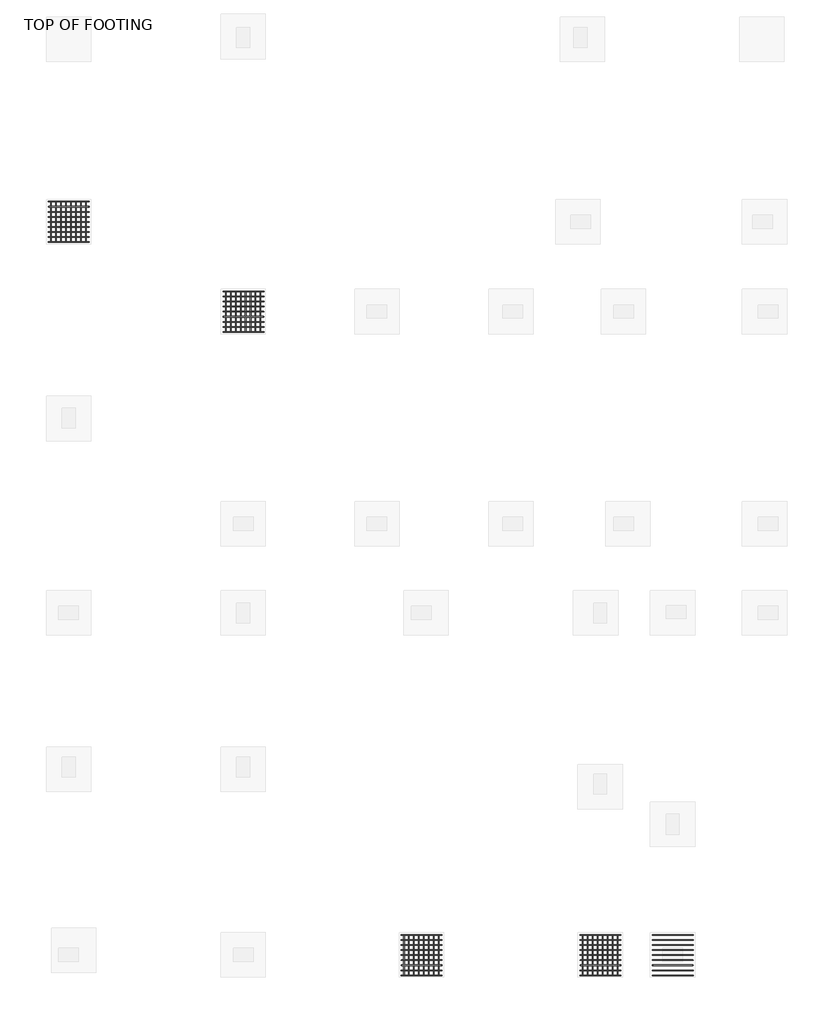
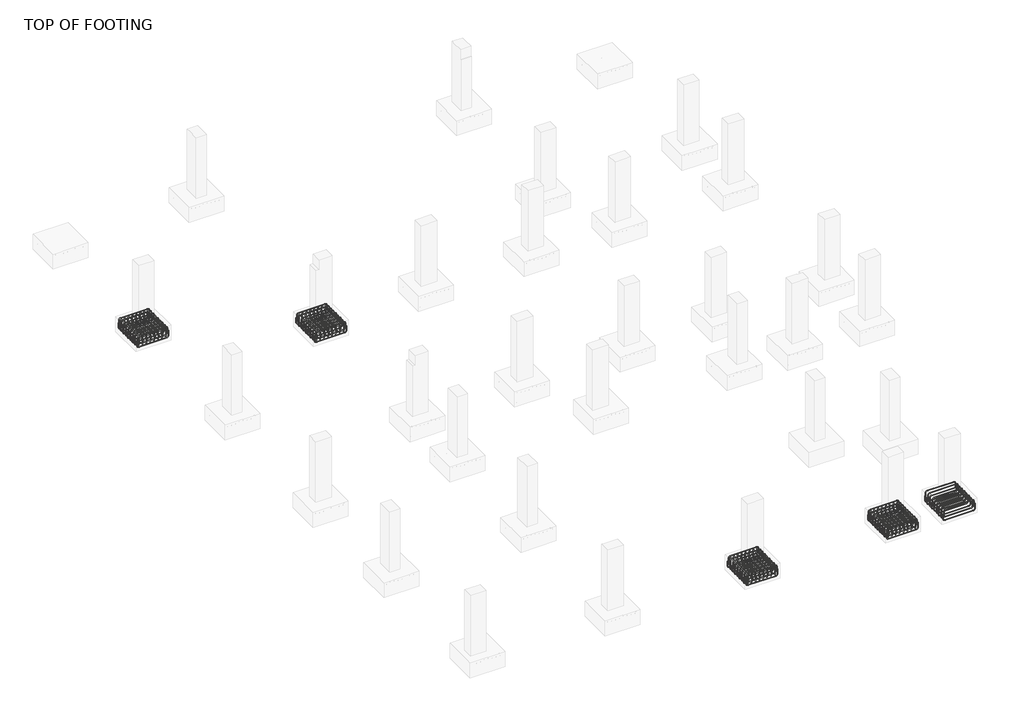
# One storey, part 5 of 20: 18 reinforcing bars.
"""IFC4 building model written with IfcOpenShell, lengths in millimetres."""

from ifc_helpers import new_model, si_unit, point, frame, origin, place, context, project, spatial, polyline, circle_curve, trimmed, segment, composite_curve, source, transform, mapped, element, save
from ifc_brep_helpers import swept_disk

model = new_model("IFC4")

# Units and contexts
model_context = context("Model", 3, world=origin())
ifc_project = project(units=[si_unit("LENGTHUNIT", "METRE", prefix="MILLI")], contexts=[model_context])

# Site, building, storey
site = spatial("IfcSite", under=ifc_project)
building = spatial("IfcBuilding", under=site)
storey = spatial("IfcBuildingStorey", under=building, Name="TOP OF FOOTING", Elevation=-1828.8)

# Reinforcing bars
placement = place(None, origin())
reinforcing_bar_shape = source(origin(), model_context, "Body", "SolidModel", [
    swept_disk(composite_curve([segment(polyline([(-1368.1365686, -4547.9729916, -2006.6587682), (-1368.1365686, -4547.9729916, -2153.9587682)]), True, "CONTINUOUS"), segment(trimmed(circle_curve(frame((-1414.4865686, -4547.9729916, -2153.9587682), z_axis=(0.0, 1.0, 0.0), x_axis=(46.350000000000136, 0.0, 0.0)), 46.35), [point((-1368.1365686, -4547.9729916, -2153.9587682))], [point((-1414.4865686, -4547.9729916, -2200.3087682))], True, "CARTESIAN"), True, "CONTINUOUS"), segment(polyline([(-1414.4865686, -4547.9729916, -2200.3087682), (-2229.0865686, -4547.9729916, -2200.3087682)]), True, "CONTINUOUS"), segment(trimmed(circle_curve(frame((-2229.0865686, -4547.9729916, -2153.9587682), z_axis=(0.0, 1.0, 0.0), x_axis=(0.0, 0.0, -46.34999999999991)), 46.35), [point((-2229.0865686, -4547.9729916, -2200.3087682))], [point((-2275.4365686, -4547.9729916, -2153.9587682))], True, "CARTESIAN"), True, "CONTINUOUS"), segment(polyline([(-2275.4365686, -4547.9729916, -2153.9587682), (-2275.4365686, -4547.9729916, -2006.6587682)]), True, "CONTINUOUS")], self_intersect=False), 6.35),
])
element("IfcReinforcingBar", 1, at=placement, inside=storey, context=model_context, shape_type="MappedRepresentation", body=[
    mapped(reinforcing_bar_shape, transform((0.0, 0.0, 0.0), x_axis=(1.0, 0.0, 0.0), y_axis=(0.0, 1.0, 0.0), z_axis=(0.0, 0.0, 1.0))),
    mapped(reinforcing_bar_shape, transform((0.0, -113.4125, 0.0), x_axis=(1.0, 0.0, 0.0), y_axis=(0.0, 1.0, 0.0), z_axis=(0.0, 0.0, 1.0))),
    mapped(reinforcing_bar_shape, transform((0.0, -226.825, 0.0), x_axis=(1.0, 0.0, 0.0), y_axis=(0.0, 1.0, 0.0), z_axis=(0.0, 0.0, 1.0))),
    mapped(reinforcing_bar_shape, transform((0.0, -340.2375, 0.0), x_axis=(1.0, 0.0, 0.0), y_axis=(0.0, 1.0, 0.0), z_axis=(0.0, 0.0, 1.0))),
    mapped(reinforcing_bar_shape, transform((0.0, -453.65, 0.0), x_axis=(1.0, 0.0, 0.0), y_axis=(0.0, 1.0, 0.0), z_axis=(0.0, 0.0, 1.0))),
    mapped(reinforcing_bar_shape, transform((0.0, -567.0625, 0.0), x_axis=(1.0, 0.0, 0.0), y_axis=(0.0, 1.0, 0.0), z_axis=(0.0, 0.0, 1.0))),
    mapped(reinforcing_bar_shape, transform((0.0, -680.475, 0.0), x_axis=(1.0, 0.0, 0.0), y_axis=(0.0, 1.0, 0.0), z_axis=(0.0, 0.0, 1.0))),
    mapped(reinforcing_bar_shape, transform((0.0, -793.8875, 0.0), x_axis=(1.0, 0.0, 0.0), y_axis=(0.0, 1.0, 0.0), z_axis=(0.0, 0.0, 1.0))),
    mapped(reinforcing_bar_shape, transform((0.0, -907.3, 0.0), x_axis=(1.0, 0.0, 0.0), y_axis=(0.0, 1.0, 0.0), z_axis=(0.0, 0.0, 1.0))),
])
reinforcing_bar_2_shape = source(origin(), model_context, "Body", "SolidModel", [
    swept_disk(composite_curve([segment(polyline([(-2255.9624573, -4547.9729916, -2068.8), (-2255.9624573, -4547.9729916, -1921.5)]), True, "CONTINUOUS"), segment(trimmed(circle_curve(frame((-2209.6124573, -4547.9729916, -1921.5), z_axis=(0.0, 1.0, 0.0), x_axis=(-46.34999999999991, 0.0, 0.0)), 46.35), [point((-2255.9624573, -4547.9729916, -1921.5))], [point((-2209.6124573, -4547.9729916, -1875.15))], True, "CARTESIAN"), True, "CONTINUOUS"), segment(polyline([(-2209.6124573, -4547.9729916, -1875.15), (-1440.1490576, -4547.9729916, -1875.15)]), True, "CONTINUOUS"), segment(trimmed(circle_curve(frame((-1440.1490576, -4547.9729916, -1921.5), z_axis=(0.0, 1.0, 0.0), x_axis=(0.0, 0.0, 46.34999999999991)), 46.35), [point((-1440.1490576, -4547.9729916, -1875.15))], [point((-1393.7990576, -4547.9729916, -1921.5))], True, "CARTESIAN"), True, "CONTINUOUS"), segment(polyline([(-1393.7990576, -4547.9729916, -1921.5), (-1393.7990576, -4547.9729916, -2068.8)]), True, "CONTINUOUS")], self_intersect=False), 6.35),
])
element("IfcReinforcingBar", 2, at=placement, inside=storey, context=model_context, shape_type="MappedRepresentation", body=[
    mapped(reinforcing_bar_2_shape, transform((0.0, 0.0, 0.0), x_axis=(1.0, 0.0, 0.0), y_axis=(0.0, 1.0, 0.0), z_axis=(0.0, 0.0, 1.0))),
    mapped(reinforcing_bar_2_shape, transform((0.0, -113.4125, 0.0), x_axis=(1.0, 0.0, 0.0), y_axis=(0.0, 1.0, 0.0), z_axis=(0.0, 0.0, 1.0))),
    mapped(reinforcing_bar_2_shape, transform((0.0, -226.825, 0.0), x_axis=(1.0, 0.0, 0.0), y_axis=(0.0, 1.0, 0.0), z_axis=(0.0, 0.0, 1.0))),
    mapped(reinforcing_bar_2_shape, transform((0.0, -340.2375, 0.0), x_axis=(1.0, 0.0, 0.0), y_axis=(0.0, 1.0, 0.0), z_axis=(0.0, 0.0, 1.0))),
    mapped(reinforcing_bar_2_shape, transform((0.0, -453.65, 0.0), x_axis=(1.0, 0.0, 0.0), y_axis=(0.0, 1.0, 0.0), z_axis=(0.0, 0.0, 1.0))),
    mapped(reinforcing_bar_2_shape, transform((0.0, -567.0625, 0.0), x_axis=(1.0, 0.0, 0.0), y_axis=(0.0, 1.0, 0.0), z_axis=(0.0, 0.0, 1.0))),
    mapped(reinforcing_bar_2_shape, transform((0.0, -680.475, 0.0), x_axis=(1.0, 0.0, 0.0), y_axis=(0.0, 1.0, 0.0), z_axis=(0.0, 0.0, 1.0))),
    mapped(reinforcing_bar_2_shape, transform((0.0, -793.8875, 0.0), x_axis=(1.0, 0.0, 0.0), y_axis=(0.0, 1.0, 0.0), z_axis=(0.0, 0.0, 1.0))),
    mapped(reinforcing_bar_2_shape, transform((0.0, -907.3, 0.0), x_axis=(1.0, 0.0, 0.0), y_axis=(0.0, 1.0, 0.0), z_axis=(0.0, 0.0, 1.0))),
])
reinforcing_bar_3_shape = source(origin(), model_context, "Body", "SolidModel", [
    swept_disk(composite_curve([segment(polyline([(-1439.63353, -4547.9729916, -2086.1951968), (-1439.63353, -4547.9729916, -1938.8951968)]), True, "CONTINUOUS"), segment(trimmed(circle_curve(frame((-1439.63353, -4594.3229916, -1938.8951968), z_axis=(1.0, 0.0, 0.0), x_axis=(0.0, 46.350000000000364, 0.0)), 46.35), [point((-1439.63353, -4547.9729916, -1938.8951968))], [point((-1439.63353, -4594.3229916, -1892.5451968))], True, "CARTESIAN"), True, "CONTINUOUS"), segment(polyline([(-1439.63353, -4594.3229916, -1892.5451968), (-1439.63353, -5408.9229916, -1892.5451968)]), True, "CONTINUOUS"), segment(trimmed(circle_curve(frame((-1439.63353, -5408.9229916, -1938.8951968), z_axis=(1.0, 0.0, 0.0), x_axis=(0.0, 0.0, 46.34999999999991)), 46.35), [point((-1439.63353, -5408.9229916, -1892.5451968))], [point((-1439.63353, -5455.2729916, -1938.8951968))], True, "CARTESIAN"), True, "CONTINUOUS"), segment(polyline([(-1439.63353, -5455.2729916, -1938.8951968), (-1439.63353, -5455.2729916, -2086.1951968)]), True, "CONTINUOUS")], self_intersect=False), 6.35),
])
element("IfcReinforcingBar", 3, at=placement, inside=storey, context=model_context, shape_type="MappedRepresentation", body=[
    mapped(reinforcing_bar_3_shape, transform((0.0, 0.0, 0.0), x_axis=(1.0, 0.0, 0.0), y_axis=(0.0, 1.0, 0.0), z_axis=(0.0, 0.0, 1.0))),
    mapped(reinforcing_bar_3_shape, transform((-111.2862402, 0.0, 0.0), x_axis=(1.0, 0.0, 0.0), y_axis=(0.0, 1.0, 0.0), z_axis=(0.0, 0.0, 1.0))),
    mapped(reinforcing_bar_3_shape, transform((-222.5724804, 0.0, 0.0), x_axis=(1.0, 0.0, 0.0), y_axis=(0.0, 1.0, 0.0), z_axis=(0.0, 0.0, 1.0))),
    mapped(reinforcing_bar_3_shape, transform((-333.8587205, 0.0, 0.0), x_axis=(1.0, 0.0, 0.0), y_axis=(0.0, 1.0, 0.0), z_axis=(0.0, 0.0, 1.0))),
    mapped(reinforcing_bar_3_shape, transform((-445.1449607, 0.0, 0.0), x_axis=(1.0, 0.0, 0.0), y_axis=(0.0, 1.0, 0.0), z_axis=(0.0, 0.0, 1.0))),
    mapped(reinforcing_bar_3_shape, transform((-556.4312009, 0.0, 0.0), x_axis=(1.0, 0.0, 0.0), y_axis=(0.0, 1.0, 0.0), z_axis=(0.0, 0.0, 1.0))),
    mapped(reinforcing_bar_3_shape, transform((-667.7174411, 0.0, 0.0), x_axis=(1.0, 0.0, 0.0), y_axis=(0.0, 1.0, 0.0), z_axis=(0.0, 0.0, 1.0))),
    mapped(reinforcing_bar_3_shape, transform((-779.0036813, 0.0, 0.0), x_axis=(1.0, 0.0, 0.0), y_axis=(0.0, 1.0, 0.0), z_axis=(0.0, 0.0, 1.0))),
])
reinforcing_bar_4_shape = source(origin(), model_context, "Body", "SolidModel", [
    swept_disk(composite_curve([segment(polyline([(-2218.6372113, -4547.9729916, -1979.1645013), (-2218.6372113, -4547.9729916, -2126.4645013)]), True, "CONTINUOUS"), segment(trimmed(circle_curve(frame((-2218.6372113, -4594.3229916, -2126.4645013), z_axis=(-1.0, 0.0, 0.0), x_axis=(0.0, 46.350000000000364, 0.0)), 46.35), [point((-2218.6372113, -4547.9729916, -2126.4645013))], [point((-2218.6372113, -4594.3229916, -2172.8145013))], True, "CARTESIAN"), True, "CONTINUOUS"), segment(polyline([(-2218.6372113, -4594.3229916, -2172.8145013), (-2218.6372113, -5408.9229916, -2172.8145013)]), True, "CONTINUOUS"), segment(trimmed(circle_curve(frame((-2218.6372113, -5408.9229916, -2126.4645013), z_axis=(-1.0, 0.0, 0.0), x_axis=(0.0, 0.0, -46.34999999999991)), 46.35), [point((-2218.6372113, -5408.9229916, -2172.8145013))], [point((-2218.6372113, -5455.2729916, -2126.4645013))], True, "CARTESIAN"), True, "CONTINUOUS"), segment(polyline([(-2218.6372113, -5455.2729916, -2126.4645013), (-2218.6372113, -5455.2729916, -1979.1645013)]), True, "CONTINUOUS")], self_intersect=False), 6.35),
])
element("IfcReinforcingBar", 4, at=placement, inside=storey, context=model_context, shape_type="MappedRepresentation", body=[
    mapped(reinforcing_bar_4_shape, transform((0.0, 0.0, 0.0), x_axis=(1.0, 0.0, 0.0), y_axis=(0.0, 1.0, 0.0), z_axis=(0.0, 0.0, 1.0))),
    mapped(reinforcing_bar_4_shape, transform((111.2862402, 0.0, 0.0), x_axis=(1.0, 0.0, 0.0), y_axis=(0.0, 1.0, 0.0), z_axis=(0.0, 0.0, 1.0))),
    mapped(reinforcing_bar_4_shape, transform((222.5724804, 0.0, 0.0), x_axis=(1.0, 0.0, 0.0), y_axis=(0.0, 1.0, 0.0), z_axis=(0.0, 0.0, 1.0))),
    mapped(reinforcing_bar_4_shape, transform((333.8587205, 0.0, 0.0), x_axis=(1.0, 0.0, 0.0), y_axis=(0.0, 1.0, 0.0), z_axis=(0.0, 0.0, 1.0))),
    mapped(reinforcing_bar_4_shape, transform((445.1449607, 0.0, 0.0), x_axis=(1.0, 0.0, 0.0), y_axis=(0.0, 1.0, 0.0), z_axis=(0.0, 0.0, 1.0))),
    mapped(reinforcing_bar_4_shape, transform((556.4312009, 0.0, 0.0), x_axis=(1.0, 0.0, 0.0), y_axis=(0.0, 1.0, 0.0), z_axis=(0.0, 0.0, 1.0))),
    mapped(reinforcing_bar_4_shape, transform((667.7174411, 0.0, 0.0), x_axis=(1.0, 0.0, 0.0), y_axis=(0.0, 1.0, 0.0), z_axis=(0.0, 0.0, 1.0))),
    mapped(reinforcing_bar_4_shape, transform((779.0036813, 0.0, 0.0), x_axis=(1.0, 0.0, 0.0), y_axis=(0.0, 1.0, 0.0), z_axis=(0.0, 0.0, 1.0))),
])
reinforcing_bar_5_shape = source(origin(), model_context, "Body", "SolidModel", [
    swept_disk(composite_curve([segment(polyline([(-5285.1605653, -2535.8035766, -2006.6587682), (-5285.1605653, -2535.8035766, -2153.9587682)]), True, "CONTINUOUS"), segment(trimmed(circle_curve(frame((-5331.5105653, -2535.8035766, -2153.9587682), z_axis=(0.0, 1.0, 0.0), x_axis=(46.350000000000364, 0.0, 0.0)), 46.35), [point((-5285.1605653, -2535.8035766, -2153.9587682))], [point((-5331.5105653, -2535.8035766, -2200.3087682))], True, "CARTESIAN"), True, "CONTINUOUS"), segment(polyline([(-5331.5105653, -2535.8035766, -2200.3087682), (-6146.1105653, -2535.8035766, -2200.3087682)]), True, "CONTINUOUS"), segment(trimmed(circle_curve(frame((-6146.1105653, -2535.8035766, -2153.9587682), z_axis=(0.0, 1.0, 0.0), x_axis=(0.0, 0.0, -46.34999999999991)), 46.35), [point((-6146.1105653, -2535.8035766, -2200.3087682))], [point((-6192.4605653, -2535.8035766, -2153.9587682))], True, "CARTESIAN"), True, "CONTINUOUS"), segment(polyline([(-6192.4605653, -2535.8035766, -2153.9587682), (-6192.4605653, -2535.8035766, -2006.6587682)]), True, "CONTINUOUS")], self_intersect=False), 6.35),
])
element("IfcReinforcingBar", 5, at=placement, inside=storey, context=model_context, shape_type="MappedRepresentation", body=[
    mapped(reinforcing_bar_5_shape, transform((0.0, 0.0, 0.0), x_axis=(1.0, 0.0, 0.0), y_axis=(0.0, 1.0, 0.0), z_axis=(0.0, 0.0, 1.0))),
    mapped(reinforcing_bar_5_shape, transform((0.0, -113.4125, 0.0), x_axis=(1.0, 0.0, 0.0), y_axis=(0.0, 1.0, 0.0), z_axis=(0.0, 0.0, 1.0))),
    mapped(reinforcing_bar_5_shape, transform((0.0, -226.825, 0.0), x_axis=(1.0, 0.0, 0.0), y_axis=(0.0, 1.0, 0.0), z_axis=(0.0, 0.0, 1.0))),
    mapped(reinforcing_bar_5_shape, transform((0.0, -340.2375, 0.0), x_axis=(1.0, 0.0, 0.0), y_axis=(0.0, 1.0, 0.0), z_axis=(0.0, 0.0, 1.0))),
    mapped(reinforcing_bar_5_shape, transform((0.0, -453.65, 0.0), x_axis=(1.0, 0.0, 0.0), y_axis=(0.0, 1.0, 0.0), z_axis=(0.0, 0.0, 1.0))),
    mapped(reinforcing_bar_5_shape, transform((0.0, -567.0625, 0.0), x_axis=(1.0, 0.0, 0.0), y_axis=(0.0, 1.0, 0.0), z_axis=(0.0, 0.0, 1.0))),
    mapped(reinforcing_bar_5_shape, transform((0.0, -680.475, 0.0), x_axis=(1.0, 0.0, 0.0), y_axis=(0.0, 1.0, 0.0), z_axis=(0.0, 0.0, 1.0))),
    mapped(reinforcing_bar_5_shape, transform((0.0, -793.8875, 0.0), x_axis=(1.0, 0.0, 0.0), y_axis=(0.0, 1.0, 0.0), z_axis=(0.0, 0.0, 1.0))),
    mapped(reinforcing_bar_5_shape, transform((0.0, -907.3, 0.0), x_axis=(1.0, 0.0, 0.0), y_axis=(0.0, 1.0, 0.0), z_axis=(0.0, 0.0, 1.0))),
])
reinforcing_bar_6_shape = source(origin(), model_context, "Body", "SolidModel", [
    swept_disk(composite_curve([segment(polyline([(-6172.986454, -2535.8035766, -2068.8), (-6172.986454, -2535.8035766, -1921.5)]), True, "CONTINUOUS"), segment(trimmed(circle_curve(frame((-6126.636454, -2535.8035766, -1921.5), z_axis=(0.0, 1.0, 0.0), x_axis=(-46.349999999999454, 0.0, 0.0)), 46.35), [point((-6172.986454, -2535.8035766, -1921.5))], [point((-6126.636454, -2535.8035766, -1875.15))], True, "CARTESIAN"), True, "CONTINUOUS"), segment(polyline([(-6126.636454, -2535.8035766, -1875.15), (-5357.1730543, -2535.8035766, -1875.15)]), True, "CONTINUOUS"), segment(trimmed(circle_curve(frame((-5357.1730543, -2535.8035766, -1921.5), z_axis=(0.0, 1.0, 0.0), x_axis=(0.0, 0.0, 46.34999999999991)), 46.35), [point((-5357.1730543, -2535.8035766, -1875.15))], [point((-5310.8230543, -2535.8035766, -1921.5))], True, "CARTESIAN"), True, "CONTINUOUS"), segment(polyline([(-5310.8230543, -2535.8035766, -1921.5), (-5310.8230543, -2535.8035766, -2068.8)]), True, "CONTINUOUS")], self_intersect=False), 6.35),
])
element("IfcReinforcingBar", 6, at=placement, inside=storey, context=model_context, shape_type="MappedRepresentation", body=[
    mapped(reinforcing_bar_6_shape, transform((0.0, 0.0, 0.0), x_axis=(1.0, 0.0, 0.0), y_axis=(0.0, 1.0, 0.0), z_axis=(0.0, 0.0, 1.0))),
    mapped(reinforcing_bar_6_shape, transform((0.0, -113.4125, 0.0), x_axis=(1.0, 0.0, 0.0), y_axis=(0.0, 1.0, 0.0), z_axis=(0.0, 0.0, 1.0))),
    mapped(reinforcing_bar_6_shape, transform((0.0, -226.825, 0.0), x_axis=(1.0, 0.0, 0.0), y_axis=(0.0, 1.0, 0.0), z_axis=(0.0, 0.0, 1.0))),
    mapped(reinforcing_bar_6_shape, transform((0.0, -340.2375, 0.0), x_axis=(1.0, 0.0, 0.0), y_axis=(0.0, 1.0, 0.0), z_axis=(0.0, 0.0, 1.0))),
    mapped(reinforcing_bar_6_shape, transform((0.0, -453.65, 0.0), x_axis=(1.0, 0.0, 0.0), y_axis=(0.0, 1.0, 0.0), z_axis=(0.0, 0.0, 1.0))),
    mapped(reinforcing_bar_6_shape, transform((0.0, -567.0625, 0.0), x_axis=(1.0, 0.0, 0.0), y_axis=(0.0, 1.0, 0.0), z_axis=(0.0, 0.0, 1.0))),
    mapped(reinforcing_bar_6_shape, transform((0.0, -680.475, 0.0), x_axis=(1.0, 0.0, 0.0), y_axis=(0.0, 1.0, 0.0), z_axis=(0.0, 0.0, 1.0))),
    mapped(reinforcing_bar_6_shape, transform((0.0, -793.8875, 0.0), x_axis=(1.0, 0.0, 0.0), y_axis=(0.0, 1.0, 0.0), z_axis=(0.0, 0.0, 1.0))),
    mapped(reinforcing_bar_6_shape, transform((0.0, -907.3, 0.0), x_axis=(1.0, 0.0, 0.0), y_axis=(0.0, 1.0, 0.0), z_axis=(0.0, 0.0, 1.0))),
])
reinforcing_bar_7_shape = source(origin(), model_context, "Body", "SolidModel", [
    swept_disk(composite_curve([segment(polyline([(-5356.6575267, -2535.8035766, -2086.1951968), (-5356.6575267, -2535.8035766, -1938.8951968)]), True, "CONTINUOUS"), segment(trimmed(circle_curve(frame((-5356.6575267, -2582.1535766, -1938.8951968), z_axis=(1.0, 0.0, 0.0), x_axis=(0.0, 46.350000000000364, 0.0)), 46.35), [point((-5356.6575267, -2535.8035766, -1938.8951968))], [point((-5356.6575267, -2582.1535766, -1892.5451968))], True, "CARTESIAN"), True, "CONTINUOUS"), segment(polyline([(-5356.6575267, -2582.1535766, -1892.5451968), (-5356.6575267, -3396.7535766, -1892.5451968)]), True, "CONTINUOUS"), segment(trimmed(circle_curve(frame((-5356.6575267, -3396.7535766, -1938.8951968), z_axis=(1.0, 0.0, 0.0), x_axis=(0.0, 0.0, 46.34999999999991)), 46.35), [point((-5356.6575267, -3396.7535766, -1892.5451968))], [point((-5356.6575267, -3443.1035766, -1938.8951968))], True, "CARTESIAN"), True, "CONTINUOUS"), segment(polyline([(-5356.6575267, -3443.1035766, -1938.8951968), (-5356.6575267, -3443.1035766, -2086.1951968)]), True, "CONTINUOUS")], self_intersect=False), 6.35),
])
element("IfcReinforcingBar", 7, at=placement, inside=storey, context=model_context, shape_type="MappedRepresentation", body=[
    mapped(reinforcing_bar_7_shape, transform((0.0, 0.0, 0.0), x_axis=(1.0, 0.0, 0.0), y_axis=(0.0, 1.0, 0.0), z_axis=(0.0, 0.0, 1.0))),
    mapped(reinforcing_bar_7_shape, transform((-111.2862402, 0.0, 0.0), x_axis=(1.0, 0.0, 0.0), y_axis=(0.0, 1.0, 0.0), z_axis=(0.0, 0.0, 1.0))),
    mapped(reinforcing_bar_7_shape, transform((-222.5724804, 0.0, 0.0), x_axis=(1.0, 0.0, 0.0), y_axis=(0.0, 1.0, 0.0), z_axis=(0.0, 0.0, 1.0))),
    mapped(reinforcing_bar_7_shape, transform((-333.8587205, 0.0, 0.0), x_axis=(1.0, 0.0, 0.0), y_axis=(0.0, 1.0, 0.0), z_axis=(0.0, 0.0, 1.0))),
    mapped(reinforcing_bar_7_shape, transform((-445.1449607, 0.0, 0.0), x_axis=(1.0, 0.0, 0.0), y_axis=(0.0, 1.0, 0.0), z_axis=(0.0, 0.0, 1.0))),
    mapped(reinforcing_bar_7_shape, transform((-556.4312009, 0.0, 0.0), x_axis=(1.0, 0.0, 0.0), y_axis=(0.0, 1.0, 0.0), z_axis=(0.0, 0.0, 1.0))),
    mapped(reinforcing_bar_7_shape, transform((-667.7174411, 0.0, 0.0), x_axis=(1.0, 0.0, 0.0), y_axis=(0.0, 1.0, 0.0), z_axis=(0.0, 0.0, 1.0))),
    mapped(reinforcing_bar_7_shape, transform((-779.0036813, 0.0, 0.0), x_axis=(1.0, 0.0, 0.0), y_axis=(0.0, 1.0, 0.0), z_axis=(0.0, 0.0, 1.0))),
])
reinforcing_bar_8_shape = source(origin(), model_context, "Body", "SolidModel", [
    swept_disk(composite_curve([segment(polyline([(-6135.661208, -2535.8035766, -1979.1645013), (-6135.661208, -2535.8035766, -2126.4645013)]), True, "CONTINUOUS"), segment(trimmed(circle_curve(frame((-6135.661208, -2582.1535766, -2126.4645013), z_axis=(-1.0, 0.0, 0.0), x_axis=(0.0, 46.350000000000364, 0.0)), 46.35), [point((-6135.661208, -2535.8035766, -2126.4645013))], [point((-6135.661208, -2582.1535766, -2172.8145013))], True, "CARTESIAN"), True, "CONTINUOUS"), segment(polyline([(-6135.661208, -2582.1535766, -2172.8145013), (-6135.661208, -3396.7535766, -2172.8145013)]), True, "CONTINUOUS"), segment(trimmed(circle_curve(frame((-6135.661208, -3396.7535766, -2126.4645013), z_axis=(-1.0, 0.0, 0.0), x_axis=(0.0, 0.0, -46.34999999999991)), 46.35), [point((-6135.661208, -3396.7535766, -2172.8145013))], [point((-6135.661208, -3443.1035766, -2126.4645013))], True, "CARTESIAN"), True, "CONTINUOUS"), segment(polyline([(-6135.661208, -3443.1035766, -2126.4645013), (-6135.661208, -3443.1035766, -1979.1645013)]), True, "CONTINUOUS")], self_intersect=False), 6.35),
])
element("IfcReinforcingBar", 8, at=placement, inside=storey, context=model_context, shape_type="MappedRepresentation", body=[
    mapped(reinforcing_bar_8_shape, transform((0.0, 0.0, 0.0), x_axis=(1.0, 0.0, 0.0), y_axis=(0.0, 1.0, 0.0), z_axis=(0.0, 0.0, 1.0))),
    mapped(reinforcing_bar_8_shape, transform((111.2862402, 0.0, 0.0), x_axis=(1.0, 0.0, 0.0), y_axis=(0.0, 1.0, 0.0), z_axis=(0.0, 0.0, 1.0))),
    mapped(reinforcing_bar_8_shape, transform((222.5724804, 0.0, 0.0), x_axis=(1.0, 0.0, 0.0), y_axis=(0.0, 1.0, 0.0), z_axis=(0.0, 0.0, 1.0))),
    mapped(reinforcing_bar_8_shape, transform((333.8587205, 0.0, 0.0), x_axis=(1.0, 0.0, 0.0), y_axis=(0.0, 1.0, 0.0), z_axis=(0.0, 0.0, 1.0))),
    mapped(reinforcing_bar_8_shape, transform((445.1449607, 0.0, 0.0), x_axis=(1.0, 0.0, 0.0), y_axis=(0.0, 1.0, 0.0), z_axis=(0.0, 0.0, 1.0))),
    mapped(reinforcing_bar_8_shape, transform((556.4312009, 0.0, 0.0), x_axis=(1.0, 0.0, 0.0), y_axis=(0.0, 1.0, 0.0), z_axis=(0.0, 0.0, 1.0))),
    mapped(reinforcing_bar_8_shape, transform((667.7174411, 0.0, 0.0), x_axis=(1.0, 0.0, 0.0), y_axis=(0.0, 1.0, 0.0), z_axis=(0.0, 0.0, 1.0))),
    mapped(reinforcing_bar_8_shape, transform((779.0036813, 0.0, 0.0), x_axis=(1.0, 0.0, 0.0), y_axis=(0.0, 1.0, 0.0), z_axis=(0.0, 0.0, 1.0))),
])
reinforcing_bar_9_shape = source(origin(), model_context, "Body", "SolidModel", [
    swept_disk(composite_curve([segment(polyline([(2628.3796816, -18968.8804373, -2006.6587682), (2628.3796816, -18968.8804373, -2153.9587682)]), True, "CONTINUOUS"), segment(trimmed(circle_curve(frame((2582.0296816, -18968.8804373, -2153.9587682), z_axis=(0.0, 1.0, 0.0), x_axis=(46.34999999999991, 0.0, 0.0)), 46.35), [point((2628.3796816, -18968.8804373, -2153.9587682))], [point((2582.0296816, -18968.8804373, -2200.3087682))], True, "CARTESIAN"), True, "CONTINUOUS"), segment(polyline([(2582.0296816, -18968.8804373, -2200.3087682), (1767.4296816, -18968.8804373, -2200.3087682)]), True, "CONTINUOUS"), segment(trimmed(circle_curve(frame((1767.4296816, -18968.8804373, -2153.9587682), z_axis=(0.0, 1.0, 0.0), x_axis=(0.0, 0.0, -46.34999999999991)), 46.35), [point((1767.4296816, -18968.8804373, -2200.3087682))], [point((1721.0796816, -18968.8804373, -2153.9587682))], True, "CARTESIAN"), True, "CONTINUOUS"), segment(polyline([(1721.0796816, -18968.8804373, -2153.9587682), (1721.0796816, -18968.8804373, -2006.6587682)]), True, "CONTINUOUS")], self_intersect=False), 6.35),
])
element("IfcReinforcingBar", 9, at=placement, inside=storey, context=model_context, shape_type="MappedRepresentation", body=[
    mapped(reinforcing_bar_9_shape, transform((0.0, 0.0, 0.0), x_axis=(1.0, 0.0, 0.0), y_axis=(0.0, 1.0, 0.0), z_axis=(0.0, 0.0, 1.0))),
    mapped(reinforcing_bar_9_shape, transform((0.0, -113.4125, 0.0), x_axis=(1.0, 0.0, 0.0), y_axis=(0.0, 1.0, 0.0), z_axis=(0.0, 0.0, 1.0))),
    mapped(reinforcing_bar_9_shape, transform((0.0, -226.825, 0.0), x_axis=(1.0, 0.0, 0.0), y_axis=(0.0, 1.0, 0.0), z_axis=(0.0, 0.0, 1.0))),
    mapped(reinforcing_bar_9_shape, transform((0.0, -340.2375, 0.0), x_axis=(1.0, 0.0, 0.0), y_axis=(0.0, 1.0, 0.0), z_axis=(0.0, 0.0, 1.0))),
    mapped(reinforcing_bar_9_shape, transform((0.0, -453.65, 0.0), x_axis=(1.0, 0.0, 0.0), y_axis=(0.0, 1.0, 0.0), z_axis=(0.0, 0.0, 1.0))),
    mapped(reinforcing_bar_9_shape, transform((0.0, -567.0625, 0.0), x_axis=(1.0, 0.0, 0.0), y_axis=(0.0, 1.0, 0.0), z_axis=(0.0, 0.0, 1.0))),
    mapped(reinforcing_bar_9_shape, transform((0.0, -680.475, 0.0), x_axis=(1.0, 0.0, 0.0), y_axis=(0.0, 1.0, 0.0), z_axis=(0.0, 0.0, 1.0))),
    mapped(reinforcing_bar_9_shape, transform((0.0, -793.8875, 0.0), x_axis=(1.0, 0.0, 0.0), y_axis=(0.0, 1.0, 0.0), z_axis=(0.0, 0.0, 1.0))),
    mapped(reinforcing_bar_9_shape, transform((0.0, -907.3, 0.0), x_axis=(1.0, 0.0, 0.0), y_axis=(0.0, 1.0, 0.0), z_axis=(0.0, 0.0, 1.0))),
])
reinforcing_bar_10_shape = source(origin(), model_context, "Body", "SolidModel", [
    swept_disk(composite_curve([segment(polyline([(1740.553793, -18968.8804373, -2068.8), (1740.553793, -18968.8804373, -1921.5)]), True, "CONTINUOUS"), segment(trimmed(circle_curve(frame((1786.903793, -18968.8804373, -1921.5), z_axis=(0.0, 1.0, 0.0), x_axis=(-46.34999999999991, 0.0, 0.0)), 46.35), [point((1740.553793, -18968.8804373, -1921.5))], [point((1786.903793, -18968.8804373, -1875.15))], True, "CARTESIAN"), True, "CONTINUOUS"), segment(polyline([(1786.903793, -18968.8804373, -1875.15), (2556.3671926, -18968.8804373, -1875.15)]), True, "CONTINUOUS"), segment(trimmed(circle_curve(frame((2556.3671926, -18968.8804373, -1921.5), z_axis=(0.0, 1.0, 0.0), x_axis=(0.0, 0.0, 46.34999999999991)), 46.35), [point((2556.3671926, -18968.8804373, -1875.15))], [point((2602.7171926, -18968.8804373, -1921.5))], True, "CARTESIAN"), True, "CONTINUOUS"), segment(polyline([(2602.7171926, -18968.8804373, -1921.5), (2602.7171926, -18968.8804373, -2068.8)]), True, "CONTINUOUS")], self_intersect=False), 6.35),
])
element("IfcReinforcingBar", 10, at=placement, inside=storey, context=model_context, shape_type="MappedRepresentation", body=[
    mapped(reinforcing_bar_10_shape, transform((0.0, 0.0, 0.0), x_axis=(1.0, 0.0, 0.0), y_axis=(0.0, 1.0, 0.0), z_axis=(0.0, 0.0, 1.0))),
    mapped(reinforcing_bar_10_shape, transform((0.0, -113.4125, 0.0), x_axis=(1.0, 0.0, 0.0), y_axis=(0.0, 1.0, 0.0), z_axis=(0.0, 0.0, 1.0))),
    mapped(reinforcing_bar_10_shape, transform((0.0, -226.825, 0.0), x_axis=(1.0, 0.0, 0.0), y_axis=(0.0, 1.0, 0.0), z_axis=(0.0, 0.0, 1.0))),
    mapped(reinforcing_bar_10_shape, transform((0.0, -340.2375, 0.0), x_axis=(1.0, 0.0, 0.0), y_axis=(0.0, 1.0, 0.0), z_axis=(0.0, 0.0, 1.0))),
    mapped(reinforcing_bar_10_shape, transform((0.0, -453.65, 0.0), x_axis=(1.0, 0.0, 0.0), y_axis=(0.0, 1.0, 0.0), z_axis=(0.0, 0.0, 1.0))),
    mapped(reinforcing_bar_10_shape, transform((0.0, -567.0625, 0.0), x_axis=(1.0, 0.0, 0.0), y_axis=(0.0, 1.0, 0.0), z_axis=(0.0, 0.0, 1.0))),
    mapped(reinforcing_bar_10_shape, transform((0.0, -680.475, 0.0), x_axis=(1.0, 0.0, 0.0), y_axis=(0.0, 1.0, 0.0), z_axis=(0.0, 0.0, 1.0))),
    mapped(reinforcing_bar_10_shape, transform((0.0, -793.8875, 0.0), x_axis=(1.0, 0.0, 0.0), y_axis=(0.0, 1.0, 0.0), z_axis=(0.0, 0.0, 1.0))),
    mapped(reinforcing_bar_10_shape, transform((0.0, -907.3, 0.0), x_axis=(1.0, 0.0, 0.0), y_axis=(0.0, 1.0, 0.0), z_axis=(0.0, 0.0, 1.0))),
])
reinforcing_bar_11_shape = source(origin(), model_context, "Body", "SolidModel", [
    swept_disk(composite_curve([segment(polyline([(2556.8827202, -18968.8804373, -2086.1951968), (2556.8827202, -18968.8804373, -1938.8951968)]), True, "CONTINUOUS"), segment(trimmed(circle_curve(frame((2556.8827202, -19015.2304373, -1938.8951968), z_axis=(1.0, 0.0, 0.0), x_axis=(0.0, 46.35000000000218, 0.0)), 46.35), [point((2556.8827202, -18968.8804373, -1938.8951968))], [point((2556.8827202, -19015.2304373, -1892.5451968))], True, "CARTESIAN"), True, "CONTINUOUS"), segment(polyline([(2556.8827202, -19015.2304373, -1892.5451968), (2556.8827202, -19829.8304373, -1892.5451968)]), True, "CONTINUOUS"), segment(trimmed(circle_curve(frame((2556.8827202, -19829.8304373, -1938.8951968), z_axis=(1.0, 0.0, 0.0), x_axis=(0.0, 0.0, 46.34999999999991)), 46.35), [point((2556.8827202, -19829.8304373, -1892.5451968))], [point((2556.8827202, -19876.1804373, -1938.8951968))], True, "CARTESIAN"), True, "CONTINUOUS"), segment(polyline([(2556.8827202, -19876.1804373, -1938.8951968), (2556.8827202, -19876.1804373, -2086.1951968)]), True, "CONTINUOUS")], self_intersect=False), 6.35),
])
element("IfcReinforcingBar", 11, at=placement, inside=storey, context=model_context, shape_type="MappedRepresentation", body=[
    mapped(reinforcing_bar_11_shape, transform((0.0, 0.0, 0.0), x_axis=(1.0, 0.0, 0.0), y_axis=(0.0, 1.0, 0.0), z_axis=(0.0, 0.0, 1.0))),
    mapped(reinforcing_bar_11_shape, transform((-111.2862402, 0.0, 0.0), x_axis=(1.0, 0.0, 0.0), y_axis=(0.0, 1.0, 0.0), z_axis=(0.0, 0.0, 1.0))),
    mapped(reinforcing_bar_11_shape, transform((-222.5724804, 0.0, 0.0), x_axis=(1.0, 0.0, 0.0), y_axis=(0.0, 1.0, 0.0), z_axis=(0.0, 0.0, 1.0))),
    mapped(reinforcing_bar_11_shape, transform((-333.8587205, 0.0, 0.0), x_axis=(1.0, 0.0, 0.0), y_axis=(0.0, 1.0, 0.0), z_axis=(0.0, 0.0, 1.0))),
    mapped(reinforcing_bar_11_shape, transform((-445.1449607, 0.0, 0.0), x_axis=(1.0, 0.0, 0.0), y_axis=(0.0, 1.0, 0.0), z_axis=(0.0, 0.0, 1.0))),
    mapped(reinforcing_bar_11_shape, transform((-556.4312009, 0.0, 0.0), x_axis=(1.0, 0.0, 0.0), y_axis=(0.0, 1.0, 0.0), z_axis=(0.0, 0.0, 1.0))),
    mapped(reinforcing_bar_11_shape, transform((-667.7174411, 0.0, 0.0), x_axis=(1.0, 0.0, 0.0), y_axis=(0.0, 1.0, 0.0), z_axis=(0.0, 0.0, 1.0))),
    mapped(reinforcing_bar_11_shape, transform((-779.0036813, 0.0, 0.0), x_axis=(1.0, 0.0, 0.0), y_axis=(0.0, 1.0, 0.0), z_axis=(0.0, 0.0, 1.0))),
])
reinforcing_bar_12_shape = source(origin(), model_context, "Body", "SolidModel", [
    swept_disk(composite_curve([segment(polyline([(1777.879039, -18968.8804373, -1979.1645013), (1777.879039, -18968.8804373, -2126.4645013)]), True, "CONTINUOUS"), segment(trimmed(circle_curve(frame((1777.879039, -19015.2304373, -2126.4645013), z_axis=(-1.0, 0.0, 0.0), x_axis=(0.0, 46.35000000000218, 0.0)), 46.35), [point((1777.879039, -18968.8804373, -2126.4645013))], [point((1777.879039, -19015.2304373, -2172.8145013))], True, "CARTESIAN"), True, "CONTINUOUS"), segment(polyline([(1777.879039, -19015.2304373, -2172.8145013), (1777.879039, -19829.8304373, -2172.8145013)]), True, "CONTINUOUS"), segment(trimmed(circle_curve(frame((1777.879039, -19829.8304373, -2126.4645013), z_axis=(-1.0, 0.0, 0.0), x_axis=(0.0, 0.0, -46.34999999999991)), 46.35), [point((1777.879039, -19829.8304373, -2172.8145013))], [point((1777.879039, -19876.1804373, -2126.4645013))], True, "CARTESIAN"), True, "CONTINUOUS"), segment(polyline([(1777.879039, -19876.1804373, -2126.4645013), (1777.879039, -19876.1804373, -1979.1645013)]), True, "CONTINUOUS")], self_intersect=False), 6.35),
])
element("IfcReinforcingBar", 12, at=placement, inside=storey, context=model_context, shape_type="MappedRepresentation", body=[
    mapped(reinforcing_bar_12_shape, transform((0.0, 0.0, 0.0), x_axis=(1.0, 0.0, 0.0), y_axis=(0.0, 1.0, 0.0), z_axis=(0.0, 0.0, 1.0))),
    mapped(reinforcing_bar_12_shape, transform((111.2862402, 0.0, 0.0), x_axis=(1.0, 0.0, 0.0), y_axis=(0.0, 1.0, 0.0), z_axis=(0.0, 0.0, 1.0))),
    mapped(reinforcing_bar_12_shape, transform((222.5724804, 0.0, 0.0), x_axis=(1.0, 0.0, 0.0), y_axis=(0.0, 1.0, 0.0), z_axis=(0.0, 0.0, 1.0))),
    mapped(reinforcing_bar_12_shape, transform((333.8587205, 0.0, 0.0), x_axis=(1.0, 0.0, 0.0), y_axis=(0.0, 1.0, 0.0), z_axis=(0.0, 0.0, 1.0))),
    mapped(reinforcing_bar_12_shape, transform((445.1449607, 0.0, 0.0), x_axis=(1.0, 0.0, 0.0), y_axis=(0.0, 1.0, 0.0), z_axis=(0.0, 0.0, 1.0))),
    mapped(reinforcing_bar_12_shape, transform((556.4312009, 0.0, 0.0), x_axis=(1.0, 0.0, 0.0), y_axis=(0.0, 1.0, 0.0), z_axis=(0.0, 0.0, 1.0))),
    mapped(reinforcing_bar_12_shape, transform((667.7174411, 0.0, 0.0), x_axis=(1.0, 0.0, 0.0), y_axis=(0.0, 1.0, 0.0), z_axis=(0.0, 0.0, 1.0))),
    mapped(reinforcing_bar_12_shape, transform((779.0036813, 0.0, 0.0), x_axis=(1.0, 0.0, 0.0), y_axis=(0.0, 1.0, 0.0), z_axis=(0.0, 0.0, 1.0))),
])
reinforcing_bar_13_shape = source(origin(), model_context, "Body", "SolidModel", [
    swept_disk(composite_curve([segment(polyline([(6636.1748054, -18968.8804373, -2006.6587682), (6636.1748054, -18968.8804373, -2153.9587682)]), True, "CONTINUOUS"), segment(trimmed(circle_curve(frame((6589.8248054, -18968.8804373, -2153.9587682), z_axis=(0.0, 1.0, 0.0), x_axis=(46.350000000000364, 0.0, 0.0)), 46.35), [point((6636.1748054, -18968.8804373, -2153.9587682))], [point((6589.8248054, -18968.8804373, -2200.3087682))], True, "CARTESIAN"), True, "CONTINUOUS"), segment(polyline([(6589.8248054, -18968.8804373, -2200.3087682), (5775.2248054, -18968.8804373, -2200.3087682)]), True, "CONTINUOUS"), segment(trimmed(circle_curve(frame((5775.2248054, -18968.8804373, -2153.9587682), z_axis=(0.0, 1.0, 0.0), x_axis=(0.0, 0.0, -46.34999999999991)), 46.35), [point((5775.2248054, -18968.8804373, -2200.3087682))], [point((5728.8748054, -18968.8804373, -2153.9587682))], True, "CARTESIAN"), True, "CONTINUOUS"), segment(polyline([(5728.8748054, -18968.8804373, -2153.9587682), (5728.8748054, -18968.8804373, -2006.6587682)]), True, "CONTINUOUS")], self_intersect=False), 6.35),
])
element("IfcReinforcingBar", 13, at=placement, inside=storey, context=model_context, shape_type="MappedRepresentation", body=[
    mapped(reinforcing_bar_13_shape, transform((0.0, 0.0, 0.0), x_axis=(1.0, 0.0, 0.0), y_axis=(0.0, 1.0, 0.0), z_axis=(0.0, 0.0, 1.0))),
    mapped(reinforcing_bar_13_shape, transform((0.0, -113.4125, 0.0), x_axis=(1.0, 0.0, 0.0), y_axis=(0.0, 1.0, 0.0), z_axis=(0.0, 0.0, 1.0))),
    mapped(reinforcing_bar_13_shape, transform((0.0, -226.825, 0.0), x_axis=(1.0, 0.0, 0.0), y_axis=(0.0, 1.0, 0.0), z_axis=(0.0, 0.0, 1.0))),
    mapped(reinforcing_bar_13_shape, transform((0.0, -340.2375, 0.0), x_axis=(1.0, 0.0, 0.0), y_axis=(0.0, 1.0, 0.0), z_axis=(0.0, 0.0, 1.0))),
    mapped(reinforcing_bar_13_shape, transform((0.0, -453.65, 0.0), x_axis=(1.0, 0.0, 0.0), y_axis=(0.0, 1.0, 0.0), z_axis=(0.0, 0.0, 1.0))),
    mapped(reinforcing_bar_13_shape, transform((0.0, -567.0625, 0.0), x_axis=(1.0, 0.0, 0.0), y_axis=(0.0, 1.0, 0.0), z_axis=(0.0, 0.0, 1.0))),
    mapped(reinforcing_bar_13_shape, transform((0.0, -680.475, 0.0), x_axis=(1.0, 0.0, 0.0), y_axis=(0.0, 1.0, 0.0), z_axis=(0.0, 0.0, 1.0))),
    mapped(reinforcing_bar_13_shape, transform((0.0, -793.8875, 0.0), x_axis=(1.0, 0.0, 0.0), y_axis=(0.0, 1.0, 0.0), z_axis=(0.0, 0.0, 1.0))),
    mapped(reinforcing_bar_13_shape, transform((0.0, -907.3, 0.0), x_axis=(1.0, 0.0, 0.0), y_axis=(0.0, 1.0, 0.0), z_axis=(0.0, 0.0, 1.0))),
])
reinforcing_bar_14_shape = source(origin(), model_context, "Body", "SolidModel", [
    swept_disk(composite_curve([segment(polyline([(5748.3489167, -18968.8804373, -2068.8), (5748.3489167, -18968.8804373, -1921.5)]), True, "CONTINUOUS"), segment(trimmed(circle_curve(frame((5794.6989167, -18968.8804373, -1921.5), z_axis=(0.0, 1.0, 0.0), x_axis=(-46.350000000000364, 0.0, 0.0)), 46.35), [point((5748.3489167, -18968.8804373, -1921.5))], [point((5794.6989167, -18968.8804373, -1875.15))], True, "CARTESIAN"), True, "CONTINUOUS"), segment(polyline([(5794.6989167, -18968.8804373, -1875.15), (6564.1623164, -18968.8804373, -1875.15)]), True, "CONTINUOUS"), segment(trimmed(circle_curve(frame((6564.1623164, -18968.8804373, -1921.5), z_axis=(0.0, 1.0, 0.0), x_axis=(0.0, 0.0, 46.34999999999991)), 46.35), [point((6564.1623164, -18968.8804373, -1875.15))], [point((6610.5123164, -18968.8804373, -1921.5))], True, "CARTESIAN"), True, "CONTINUOUS"), segment(polyline([(6610.5123164, -18968.8804373, -1921.5), (6610.5123164, -18968.8804373, -2068.8)]), True, "CONTINUOUS")], self_intersect=False), 6.35),
])
element("IfcReinforcingBar", 14, at=placement, inside=storey, context=model_context, shape_type="MappedRepresentation", body=[
    mapped(reinforcing_bar_14_shape, transform((0.0, 0.0, 0.0), x_axis=(1.0, 0.0, 0.0), y_axis=(0.0, 1.0, 0.0), z_axis=(0.0, 0.0, 1.0))),
    mapped(reinforcing_bar_14_shape, transform((0.0, -113.4125, 0.0), x_axis=(1.0, 0.0, 0.0), y_axis=(0.0, 1.0, 0.0), z_axis=(0.0, 0.0, 1.0))),
    mapped(reinforcing_bar_14_shape, transform((0.0, -226.825, 0.0), x_axis=(1.0, 0.0, 0.0), y_axis=(0.0, 1.0, 0.0), z_axis=(0.0, 0.0, 1.0))),
    mapped(reinforcing_bar_14_shape, transform((0.0, -340.2375, 0.0), x_axis=(1.0, 0.0, 0.0), y_axis=(0.0, 1.0, 0.0), z_axis=(0.0, 0.0, 1.0))),
    mapped(reinforcing_bar_14_shape, transform((0.0, -453.65, 0.0), x_axis=(1.0, 0.0, 0.0), y_axis=(0.0, 1.0, 0.0), z_axis=(0.0, 0.0, 1.0))),
    mapped(reinforcing_bar_14_shape, transform((0.0, -567.0625, 0.0), x_axis=(1.0, 0.0, 0.0), y_axis=(0.0, 1.0, 0.0), z_axis=(0.0, 0.0, 1.0))),
    mapped(reinforcing_bar_14_shape, transform((0.0, -680.475, 0.0), x_axis=(1.0, 0.0, 0.0), y_axis=(0.0, 1.0, 0.0), z_axis=(0.0, 0.0, 1.0))),
    mapped(reinforcing_bar_14_shape, transform((0.0, -793.8875, 0.0), x_axis=(1.0, 0.0, 0.0), y_axis=(0.0, 1.0, 0.0), z_axis=(0.0, 0.0, 1.0))),
    mapped(reinforcing_bar_14_shape, transform((0.0, -907.3, 0.0), x_axis=(1.0, 0.0, 0.0), y_axis=(0.0, 1.0, 0.0), z_axis=(0.0, 0.0, 1.0))),
])
reinforcing_bar_15_shape = source(origin(), model_context, "Body", "SolidModel", [
    swept_disk(composite_curve([segment(polyline([(6564.677844, -18968.8804373, -2086.1951968), (6564.677844, -18968.8804373, -1938.8951968)]), True, "CONTINUOUS"), segment(trimmed(circle_curve(frame((6564.677844, -19015.2304373, -1938.8951968), z_axis=(1.0, 0.0, 0.0), x_axis=(0.0, 46.35000000000218, 0.0)), 46.35), [point((6564.677844, -18968.8804373, -1938.8951968))], [point((6564.677844, -19015.2304373, -1892.5451968))], True, "CARTESIAN"), True, "CONTINUOUS"), segment(polyline([(6564.677844, -19015.2304373, -1892.5451968), (6564.677844, -19829.8304373, -1892.5451968)]), True, "CONTINUOUS"), segment(trimmed(circle_curve(frame((6564.677844, -19829.8304373, -1938.8951968), z_axis=(1.0, 0.0, 0.0), x_axis=(0.0, 0.0, 46.34999999999991)), 46.35), [point((6564.677844, -19829.8304373, -1892.5451968))], [point((6564.677844, -19876.1804373, -1938.8951968))], True, "CARTESIAN"), True, "CONTINUOUS"), segment(polyline([(6564.677844, -19876.1804373, -1938.8951968), (6564.677844, -19876.1804373, -2086.1951968)]), True, "CONTINUOUS")], self_intersect=False), 6.35),
])
element("IfcReinforcingBar", 15, at=placement, inside=storey, context=model_context, shape_type="MappedRepresentation", body=[
    mapped(reinforcing_bar_15_shape, transform((0.0, 0.0, 0.0), x_axis=(1.0, 0.0, 0.0), y_axis=(0.0, 1.0, 0.0), z_axis=(0.0, 0.0, 1.0))),
    mapped(reinforcing_bar_15_shape, transform((-111.2862402, 0.0, 0.0), x_axis=(1.0, 0.0, 0.0), y_axis=(0.0, 1.0, 0.0), z_axis=(0.0, 0.0, 1.0))),
    mapped(reinforcing_bar_15_shape, transform((-222.5724804, 0.0, 0.0), x_axis=(1.0, 0.0, 0.0), y_axis=(0.0, 1.0, 0.0), z_axis=(0.0, 0.0, 1.0))),
    mapped(reinforcing_bar_15_shape, transform((-333.8587205, 0.0, 0.0), x_axis=(1.0, 0.0, 0.0), y_axis=(0.0, 1.0, 0.0), z_axis=(0.0, 0.0, 1.0))),
    mapped(reinforcing_bar_15_shape, transform((-445.1449607, 0.0, 0.0), x_axis=(1.0, 0.0, 0.0), y_axis=(0.0, 1.0, 0.0), z_axis=(0.0, 0.0, 1.0))),
    mapped(reinforcing_bar_15_shape, transform((-556.4312009, 0.0, 0.0), x_axis=(1.0, 0.0, 0.0), y_axis=(0.0, 1.0, 0.0), z_axis=(0.0, 0.0, 1.0))),
    mapped(reinforcing_bar_15_shape, transform((-667.7174411, 0.0, 0.0), x_axis=(1.0, 0.0, 0.0), y_axis=(0.0, 1.0, 0.0), z_axis=(0.0, 0.0, 1.0))),
    mapped(reinforcing_bar_15_shape, transform((-779.0036813, 0.0, 0.0), x_axis=(1.0, 0.0, 0.0), y_axis=(0.0, 1.0, 0.0), z_axis=(0.0, 0.0, 1.0))),
])
reinforcing_bar_16_shape = source(origin(), model_context, "Body", "SolidModel", [
    swept_disk(composite_curve([segment(polyline([(5785.6741627, -18968.8804373, -1979.1645013), (5785.6741627, -18968.8804373, -2126.4645013)]), True, "CONTINUOUS"), segment(trimmed(circle_curve(frame((5785.6741627, -19015.2304373, -2126.4645013), z_axis=(-1.0, 0.0, 0.0), x_axis=(0.0, 46.35000000000218, 0.0)), 46.35), [point((5785.6741627, -18968.8804373, -2126.4645013))], [point((5785.6741627, -19015.2304373, -2172.8145013))], True, "CARTESIAN"), True, "CONTINUOUS"), segment(polyline([(5785.6741627, -19015.2304373, -2172.8145013), (5785.6741627, -19829.8304373, -2172.8145013)]), True, "CONTINUOUS"), segment(trimmed(circle_curve(frame((5785.6741627, -19829.8304373, -2126.4645013), z_axis=(-1.0, 0.0, 0.0), x_axis=(0.0, 0.0, -46.34999999999991)), 46.35), [point((5785.6741627, -19829.8304373, -2172.8145013))], [point((5785.6741627, -19876.1804373, -2126.4645013))], True, "CARTESIAN"), True, "CONTINUOUS"), segment(polyline([(5785.6741627, -19876.1804373, -2126.4645013), (5785.6741627, -19876.1804373, -1979.1645013)]), True, "CONTINUOUS")], self_intersect=False), 6.35),
])
element("IfcReinforcingBar", 16, at=placement, inside=storey, context=model_context, shape_type="MappedRepresentation", body=[
    mapped(reinforcing_bar_16_shape, transform((0.0, 0.0, 0.0), x_axis=(1.0, 0.0, 0.0), y_axis=(0.0, 1.0, 0.0), z_axis=(0.0, 0.0, 1.0))),
    mapped(reinforcing_bar_16_shape, transform((111.2862402, 0.0, 0.0), x_axis=(1.0, 0.0, 0.0), y_axis=(0.0, 1.0, 0.0), z_axis=(0.0, 0.0, 1.0))),
    mapped(reinforcing_bar_16_shape, transform((222.5724804, 0.0, 0.0), x_axis=(1.0, 0.0, 0.0), y_axis=(0.0, 1.0, 0.0), z_axis=(0.0, 0.0, 1.0))),
    mapped(reinforcing_bar_16_shape, transform((333.8587205, 0.0, 0.0), x_axis=(1.0, 0.0, 0.0), y_axis=(0.0, 1.0, 0.0), z_axis=(0.0, 0.0, 1.0))),
    mapped(reinforcing_bar_16_shape, transform((445.1449607, 0.0, 0.0), x_axis=(1.0, 0.0, 0.0), y_axis=(0.0, 1.0, 0.0), z_axis=(0.0, 0.0, 1.0))),
    mapped(reinforcing_bar_16_shape, transform((556.4312009, 0.0, 0.0), x_axis=(1.0, 0.0, 0.0), y_axis=(0.0, 1.0, 0.0), z_axis=(0.0, 0.0, 1.0))),
    mapped(reinforcing_bar_16_shape, transform((667.7174411, 0.0, 0.0), x_axis=(1.0, 0.0, 0.0), y_axis=(0.0, 1.0, 0.0), z_axis=(0.0, 0.0, 1.0))),
    mapped(reinforcing_bar_16_shape, transform((779.0036813, 0.0, 0.0), x_axis=(1.0, 0.0, 0.0), y_axis=(0.0, 1.0, 0.0), z_axis=(0.0, 0.0, 1.0))),
])
reinforcing_bar_17_shape = source(origin(), model_context, "Body", "SolidModel", [
    swept_disk(composite_curve([segment(polyline([(8260.5179014, -18968.8804373, -2006.6587682), (8260.5179014, -18968.8804373, -2153.9587682)]), True, "CONTINUOUS"), segment(trimmed(circle_curve(frame((8214.1679014, -18968.8804373, -2153.9587682), z_axis=(0.0, 1.0, 0.0), x_axis=(46.350000000000364, 0.0, 0.0)), 46.35), [point((8260.5179014, -18968.8804373, -2153.9587682))], [point((8214.1679014, -18968.8804373, -2200.3087682))], True, "CARTESIAN"), True, "CONTINUOUS"), segment(polyline([(8214.1679014, -18968.8804373, -2200.3087682), (7399.5679014, -18968.8804373, -2200.3087682)]), True, "CONTINUOUS"), segment(trimmed(circle_curve(frame((7399.5679014, -18968.8804373, -2153.9587682), z_axis=(0.0, 1.0, 0.0), x_axis=(0.0, 0.0, -46.34999999999991)), 46.35), [point((7399.5679014, -18968.8804373, -2200.3087682))], [point((7353.2179014, -18968.8804373, -2153.9587682))], True, "CARTESIAN"), True, "CONTINUOUS"), segment(polyline([(7353.2179014, -18968.8804373, -2153.9587682), (7353.2179014, -18968.8804373, -2006.6587682)]), True, "CONTINUOUS")], self_intersect=False), 6.35),
])
element("IfcReinforcingBar", 17, at=placement, inside=storey, context=model_context, shape_type="MappedRepresentation", body=[
    mapped(reinforcing_bar_17_shape, transform((0.0, 0.0, 0.0), x_axis=(1.0, 0.0, 0.0), y_axis=(0.0, 1.0, 0.0), z_axis=(0.0, 0.0, 1.0))),
    mapped(reinforcing_bar_17_shape, transform((0.0, -113.4125, 0.0), x_axis=(1.0, 0.0, 0.0), y_axis=(0.0, 1.0, 0.0), z_axis=(0.0, 0.0, 1.0))),
    mapped(reinforcing_bar_17_shape, transform((0.0, -226.825, 0.0), x_axis=(1.0, 0.0, 0.0), y_axis=(0.0, 1.0, 0.0), z_axis=(0.0, 0.0, 1.0))),
    mapped(reinforcing_bar_17_shape, transform((0.0, -340.2375, 0.0), x_axis=(1.0, 0.0, 0.0), y_axis=(0.0, 1.0, 0.0), z_axis=(0.0, 0.0, 1.0))),
    mapped(reinforcing_bar_17_shape, transform((0.0, -453.65, 0.0), x_axis=(1.0, 0.0, 0.0), y_axis=(0.0, 1.0, 0.0), z_axis=(0.0, 0.0, 1.0))),
    mapped(reinforcing_bar_17_shape, transform((0.0, -567.0625, 0.0), x_axis=(1.0, 0.0, 0.0), y_axis=(0.0, 1.0, 0.0), z_axis=(0.0, 0.0, 1.0))),
    mapped(reinforcing_bar_17_shape, transform((0.0, -680.475, 0.0), x_axis=(1.0, 0.0, 0.0), y_axis=(0.0, 1.0, 0.0), z_axis=(0.0, 0.0, 1.0))),
    mapped(reinforcing_bar_17_shape, transform((0.0, -793.8875, 0.0), x_axis=(1.0, 0.0, 0.0), y_axis=(0.0, 1.0, 0.0), z_axis=(0.0, 0.0, 1.0))),
    mapped(reinforcing_bar_17_shape, transform((0.0, -907.3, 0.0), x_axis=(1.0, 0.0, 0.0), y_axis=(0.0, 1.0, 0.0), z_axis=(0.0, 0.0, 1.0))),
])
reinforcing_bar_18_shape = source(origin(), model_context, "Body", "SolidModel", [
    swept_disk(composite_curve([segment(polyline([(7372.6920127, -18968.8804373, -2068.8), (7372.6920127, -18968.8804373, -1921.5)]), True, "CONTINUOUS"), segment(trimmed(circle_curve(frame((7419.0420127, -18968.8804373, -1921.5), z_axis=(0.0, 1.0, 0.0), x_axis=(-46.349999999999454, 0.0, 0.0)), 46.35), [point((7372.6920127, -18968.8804373, -1921.5))], [point((7419.0420127, -18968.8804373, -1875.15))], True, "CARTESIAN"), True, "CONTINUOUS"), segment(polyline([(7419.0420127, -18968.8804373, -1875.15), (8188.5054124, -18968.8804373, -1875.15)]), True, "CONTINUOUS"), segment(trimmed(circle_curve(frame((8188.5054124, -18968.8804373, -1921.5), z_axis=(0.0, 1.0, 0.0), x_axis=(0.0, 0.0, 46.34999999999991)), 46.35), [point((8188.5054124, -18968.8804373, -1875.15))], [point((8234.8554124, -18968.8804373, -1921.5))], True, "CARTESIAN"), True, "CONTINUOUS"), segment(polyline([(8234.8554124, -18968.8804373, -1921.5), (8234.8554124, -18968.8804373, -2068.8)]), True, "CONTINUOUS")], self_intersect=False), 6.35),
])
element("IfcReinforcingBar", 18, at=placement, inside=storey, context=model_context, shape_type="MappedRepresentation", body=[
    mapped(reinforcing_bar_18_shape, transform((0.0, 0.0, 0.0), x_axis=(1.0, 0.0, 0.0), y_axis=(0.0, 1.0, 0.0), z_axis=(0.0, 0.0, 1.0))),
    mapped(reinforcing_bar_18_shape, transform((0.0, -113.4125, 0.0), x_axis=(1.0, 0.0, 0.0), y_axis=(0.0, 1.0, 0.0), z_axis=(0.0, 0.0, 1.0))),
    mapped(reinforcing_bar_18_shape, transform((0.0, -226.825, 0.0), x_axis=(1.0, 0.0, 0.0), y_axis=(0.0, 1.0, 0.0), z_axis=(0.0, 0.0, 1.0))),
    mapped(reinforcing_bar_18_shape, transform((0.0, -340.2375, 0.0), x_axis=(1.0, 0.0, 0.0), y_axis=(0.0, 1.0, 0.0), z_axis=(0.0, 0.0, 1.0))),
    mapped(reinforcing_bar_18_shape, transform((0.0, -453.65, 0.0), x_axis=(1.0, 0.0, 0.0), y_axis=(0.0, 1.0, 0.0), z_axis=(0.0, 0.0, 1.0))),
    mapped(reinforcing_bar_18_shape, transform((0.0, -567.0625, 0.0), x_axis=(1.0, 0.0, 0.0), y_axis=(0.0, 1.0, 0.0), z_axis=(0.0, 0.0, 1.0))),
    mapped(reinforcing_bar_18_shape, transform((0.0, -680.475, 0.0), x_axis=(1.0, 0.0, 0.0), y_axis=(0.0, 1.0, 0.0), z_axis=(0.0, 0.0, 1.0))),
    mapped(reinforcing_bar_18_shape, transform((0.0, -793.8875, 0.0), x_axis=(1.0, 0.0, 0.0), y_axis=(0.0, 1.0, 0.0), z_axis=(0.0, 0.0, 1.0))),
    mapped(reinforcing_bar_18_shape, transform((0.0, -907.3, 0.0), x_axis=(1.0, 0.0, 0.0), y_axis=(0.0, 1.0, 0.0), z_axis=(0.0, 0.0, 1.0))),
])

save(model, "model.ifc")

# Revit data of these elements
# Elements 1, 2, 3, 4, 5, 6, 7, 8, 9, 10, 11, 12, 13, 14, 15, 16, 17, 18 (IfcReinforcingBar)
#   Phase Created = New Construction
